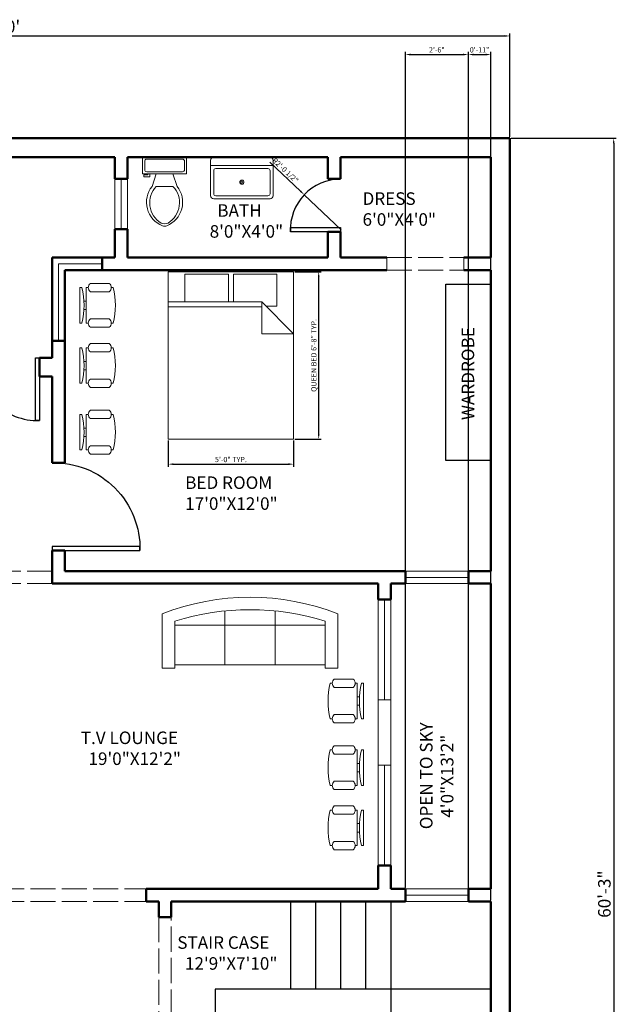
# Model space of a CAD drawing. Units: inches. Extents: x 2690 to 3266, y 1440 to 2261.
# Tile 4 of 4: x 2981 to 3266, y 1790 to 2261. Entities that reach past the tile are written whole.
import ezdxf

# ---------------------------------------------------------------- set-up
doc = ezdxf.new("R2010")
doc.units = ezdxf.units.IN
doc.linetypes.add('ACAD_ISO02W100', pattern=[15, 12, -3])
for name, color, linetype, lineweight in [('A-ANNO-DIMS', 2, 'Continuous', 18), ('A-ANNO-TEXT', 7, 'Continuous', 18), ('A-AREA-IDEN', 7, 'Continuous', 25), ('A-DOOR', 4, 'Continuous', 25), ('A-FLOR-CASE', 9, 'Continuous', 25), ('A-FLOR-FIXT', 9, 'Continuous', 18), ('A-FLOR-STRS', 7, 'Continuous', 25), ('A-FURN', 8, 'Continuous', 18), ('A-GLAZ', 3, 'Continuous', 18), ('A-WALL', 7, 'Continuous', 50), ('A-WALL-OVHD', 8, 'ACAD_ISO02W100', 18)]:
    doc.layers.add(name, color=color, linetype=linetype, lineweight=lineweight)
doc.styles.get("Standard").update_dxf_attribs({"font": 'arial.ttf'})
doc.dimstyles.new('ISO-25', dxfattribs={"dimtxt": 2.5, "dimasz": 2.5, "dimexe": 1.25, "dimexo": 0.625, "dimtad": 1, "dimlunit": 3, "dimtxsty": 'Standard', "dimcen": 2.5, "dimadec": 0, "dimazin": 0, "dimtfac": 1, "dimtmove": 0, "dimatfit": 3, "dimfxl": 1, "dimarcsym": 0})

# ---------------------------------------------------------------- blocks, each defined once
blk = doc.blocks.new('Toilet - top')
for p, q in [((9.5, -6), (9.5, -2)), ((-10, -8.5), (-8, -8.5)), ((-10, -9.5), (-10, -8.5)), ((-8, -8.5), (-8, -8)), ((-7, -8), (-7, -9.5)), ((-4, -8), (-6, -14)), ((4, -8), (6, -14)), ((-7, -9.5), (-10, -9.5)), ((4, -14), (-4, -14))]:
    blk.add_line(p, q)
blk.add_lwpolyline([(10.5, -8), (10.5, 0), (-10.5, 0), (-10.5, -8)], close=True)
for points in [[(-9.5, -2), (-9.5, -6)], [(8.5, -1), (-8.5, -1)], [(-8.5, -7), (8.5, -7)]]:
    blk.add_lwpolyline(points)
for centre, radius, start, end in [((-8.62, -1.88), 0.884, 81.8699, 188.1301), ((8.62, -1.88), 0.884, 351.8699, 98.1301), ((-8.62, -6.12), 0.884, 171.8699, 278.1301), ((8.62, -6.12), 0.884, 261.8699, 8.1301), ((3.52, -21.58), 12.17, 141.4691, 247.9714), ((4.2, -21.82), 11.33, 136.3677, 238.9468), ((-3.52, -21.58), 12.17, 292.0284, 38.5307), ((-4.2, -21.82), 11.33, 301.053, 43.6321), ((0, -27.88), 4, 245.7318, 294.2682), ((0, -29), 4, 254.8605, 285.1395)]:
    blk.add_arc(centre, radius, start, end)
blk = doc.blocks.new('Sink-single - 30 in top')
blk.add_line((-15, -3.999996), (15, -3.999996))
for points in [[(-13.5, 0), (13.5, 0)], [(-15, -18.499996), (-15, -1.5)], [(15, -1.5), (15, -18.499996)], [(-13.5, -17.499996), (-13.5, -6.499996)], [(-12.5, -5.499996), (12.5, -5.499996)], [(13.5, -6.499996), (13.5, -17.499996)], [(12.5, -18.499996), (-12.5, -18.499996)], [(13.5, -19.999996), (-13.5, -19.999996)]]:
    blk.add_lwpolyline(points)
for radius in [1, 0.5]:
    blk.add_circle((0, -11.999996), radius)
for centre, radius, start, end in [((-13.5, -1.5), 1.5, 90, 180), ((13.5, -1.5), 1.5, 0, 90), ((-12.5, -6.499996), 1, 90, 180), ((12.5, -6.499996), 1, 0, 90), ((-13.5, -18.499996), 1.5, 180, 270), ((-12.5, -17.499996), 1, 180, 270), ((12.5, -17.499996), 1, 270, 0), ((13.5, -18.499996), 1.5, 270, 0)]:
    blk.add_arc(centre, radius, start, end)
blk = doc.blocks.new('Sofa - Roundback 7 ft.')
for p, q in [((-12.00002, -32.4421), (-12.00003, -6.5971)), ((11.99997, -32.4421), (11.99998, -6.5971)), ((-36.000027, -34), (-36.000027, -11.4696)), ((-35.999844, -13.3819), (35.9998, -13.3819)), ((35.99998, -34), (35.99998, -11.4696)), ((-36.000027, -32.4421), (35.99998, -32.4421))]:
    blk.add_line(p, q)
for points in [[(-36.000027, -34), (-42.000027, -34), (-42.000027, -8)], [(41.99998, -8), (41.99998, -34), (35.99998, -34)]]:
    blk.add_lwpolyline(points)
for centre, radius, start, end in [((0, -114.25), 114.25, 68.43141, 111.5686), ((-0.00001, -127.1968), 121.1968, 72.72033, 107.2797)]:
    blk.add_arc(centre, radius, start, end)
blk = doc.blocks.new('Chair - Desk')
for p, q in [((-8.5, 0), (-8.5, -1)), ((-8.5, 0), (8.5, 0)), ((8.5, 0), (8.5, -1)), ((-8.5, -3), (-8.5, -4)), ((-8.5, -3), (8.5, -3)), ((-2, -3), (-2, -1.9355)), ((2, -1.9576), (2, -3)), ((8.5, -3), (8.5, -4)), ((-10.5, -5), (-10.5, -14)), ((-6.5, -14), (-6.5, -5)), ((6.5, -5), (6.5, -14)), ((10.5, -14), (10.5, -5)), ((-8.5, -15), (-8.5, -16)), ((8.5, -15), (8.5, -16))]:
    blk.add_line(p, q)
for centre, radius, start, end in [((-8.5, -6.5), 2.5, 36.8699, 143.1301), ((0, 34.625), 36.625, 256.5803, 283.4197), ((8.5, -6.5), 2.5, 36.8699, 143.1301), ((-8.5, -12.5), 2.5, 216.8699, 323.1301), ((8.5, -12.5), 2.5, 216.8699, 323.1301), ((0, 19.625), 36.625, 256.5803, 283.4197)]:
    blk.add_arc(centre, radius, start, end)
blk = doc.blocks.new('Bed - Queen')
for p, q in [((0, -80.00003), (0, 0)), ((0, 0), (59.99999, 0)), ((59.99999, 0), (59.99999, -80.00003)), ((7.99999, -1.2), (28.79998, -1.2)), ((7.99999, -14.4), (7.99999, -1.2)), ((28.79998, -1.2), (28.79998, -14.4)), ((31.19999, -1.2), (51.99999, -1.2)), ((31.19999, -14.4), (31.19999, -1.2)), ((51.99999, -1.2), (51.99999, -16.4)), ((0, -14.4), (44.8, -14.4)), ((44.8, -16.8), (0, -16.8)), ((59.99999, -29.6), (44.8, -14.4)), ((44.8, -14.4), (44.8, -29.6)), ((51.99999, -16.4), (46.79936, -16.4)), ((44.8, -29.6), (59.99999, -29.6)), ((59.99999, -80.00003), (0, -80.00003))]:
    blk.add_line(p, q)
blk = doc.blocks.new('*D12')
at = {"layer": 'A-ANNO-DIMS', "color": 0, "lineweight": -2, "transparency": 16777216}
for p, q in [((2735.48, 2205.11), (2735.48, 2254.67)), ((2737.98, 2253.42), (3212.98, 2253.42)), ((3215.48, 2205.11), (3215.48, 2254.67))]:
    blk.add_line(p, q, dxfattribs=at)
at = {"layer": 'A-ANNO-DIMS', "color": 0, "transparency": 16777216}
for points in [[(2737.98, 2253.84), (2737.98, 2253.01), (2735.48, 2253.42)], [(3212.98, 2253.84), (3212.98, 2253.01), (3215.48, 2253.42)]]:
    blk.add_solid(points, dxfattribs=at)
at = {"layer": 'Defpoints', "color": 0, "transparency": 16777216}
for p in [(3215.48, 2253.42), (2735.48, 2204.49), (3215.48, 2204.49)]:
    blk.add_point(p, dxfattribs=at)
at = {"layer": 'A-ANNO-DIMS', "color": 0, "transparency": 16777216, "insert": (2975.48, 2257.11), "char_height": 6, "attachment_point": 5}
blk.add_mtext("40'", dxfattribs=at)
blk = doc.blocks.new('*D15')
at = {"layer": 'A-ANNO-DIMS', "color": 0, "lineweight": -2, "transparency": 16777216}
for p, q in [((3216.1, 2204.49), (3266.46, 2204.49)), ((3265.21, 2201.99), (3265.21, 1483.99)), ((3216.1, 1481.49), (3266.46, 1481.49))]:
    blk.add_line(p, q, dxfattribs=at)
at = {"layer": 'A-ANNO-DIMS', "color": 0, "transparency": 16777216}
for points in [[(3264.79, 2201.99), (3265.63, 2201.99), (3265.21, 2204.49)], [(3264.79, 1483.99), (3265.63, 1483.99), (3265.21, 1481.49)]]:
    blk.add_solid(points, dxfattribs=at)
at = {"layer": 'Defpoints', "color": 0, "transparency": 16777216}
for p in [(3215.48, 2204.49), (3215.48, 1481.49), (3265.21, 1481.49)]:
    blk.add_point(p, dxfattribs=at)
at = {"layer": 'A-ANNO-DIMS', "color": 0, "transparency": 16777216, "insert": (3261.52, 1842.99), "char_height": 6, "attachment_point": 5, "rotation": 90}
blk.add_mtext('60\'-3"', dxfattribs=at)
blk = doc.blocks.new('DOOR-SWING-30IN')
for p, q in [((-2, -30), (-2, 0)), ((-2, 0), (0, 0)), ((0, 0), (0, -30)), ((0, -30), (-2, -30))]:
    blk.add_line(p, q)
blk.add_arc((-1, -1), 29.02, 178.0251, 271.9749)
blk = doc.blocks.new('DOOR-SWING-42IN')
for p, q in [((-42, 0), (-42, 2)), ((-42, 2), (0, 2)), ((0, 0), (-42, 0)), ((0, 2), (0, 0))]:
    blk.add_line(p, q)
blk.add_arc((-1, 1), 41.01, 88.6028, 181.3972)
blk = doc.blocks.new('WIN-24IN')
for p, q in [((0, 24), (0, 0)), ((3, 0), (3, 24)), ((3, 24), (6, 24)), ((6, 24), (6, 0)), ((0, 0), (3, 0))]:
    blk.add_line(p, q)
blk = doc.blocks.new('WARDROBE-PLAN')
blk.add_lwpolyline([(0, 0), (21.23, 0), (21.23, -84.36), (0, -84.36)], close=True)
blk = doc.blocks.new('*D29')
at = {"layer": 'A-ANNO-DIMS', "color": 0, "lineweight": -2, "transparency": 16777216}
for p, q in [((3112.66, 2140.62), (3125.28, 2140.62)), ((3124.03, 2063.12), (3124.03, 2138.12)), ((3112.66, 2060.62), (3125.28, 2060.62))]:
    blk.add_line(p, q, dxfattribs=at)
at = {"layer": 'A-ANNO-DIMS', "color": 0, "transparency": 16777216}
for points in [[(3123.61, 2138.12), (3124.45, 2138.12), (3124.03, 2140.62)], [(3123.61, 2063.12), (3124.45, 2063.12), (3124.03, 2060.62)]]:
    blk.add_solid(points, dxfattribs=at)
at = {"layer": 'Defpoints', "color": 0, "transparency": 16777216}
for p in [(3112.03, 2140.62), (3124.03, 2140.62), (3112.03, 2060.62)]:
    blk.add_point(p, dxfattribs=at)
at = {"layer": 'A-ANNO-DIMS', "color": 0, "transparency": 16777216, "insert": (3122.04, 2100.62), "char_height": 2.5, "attachment_point": 5, "rotation": 90}
blk.add_mtext('QUEEN BED 6\'-8" TYP.', dxfattribs=at)
blk = doc.blocks.new('*D30')
at = {"layer": 'A-ANNO-DIMS', "color": 0, "lineweight": -2, "transparency": 16777216}
for p, q in [((3052.03, 2059.99), (3052.03, 2047.37)), ((3112.03, 2059.99), (3112.03, 2047.37)), ((3054.53, 2048.62), (3109.53, 2048.62))]:
    blk.add_line(p, q, dxfattribs=at)
at = {"layer": 'A-ANNO-DIMS', "color": 0, "transparency": 16777216}
for points in [[(3054.53, 2049.03), (3054.53, 2048.2), (3052.03, 2048.62)], [(3109.53, 2049.03), (3109.53, 2048.2), (3112.03, 2048.62)]]:
    blk.add_solid(points, dxfattribs=at)
at = {"layer": 'Defpoints', "color": 0, "transparency": 16777216}
for p in [(3052.03, 2060.62), (3112.03, 2060.62), (3112.03, 2048.62)]:
    blk.add_point(p, dxfattribs=at)
at = {"layer": 'A-ANNO-DIMS', "color": 0, "transparency": 16777216, "insert": (3082.03, 2050.52), "char_height": 2.5, "attachment_point": 5}
blk.add_mtext('5\'-0" TYP.', dxfattribs=at)
blk = doc.blocks.new('*D58')
at = {"layer": 'A-ANNO-DIMS', "color": 0, "lineweight": -2, "transparency": 16777216}
for p, q in [((3165.5, 1846.11), (3165.5, 2245.79)), ((3168, 2244.54), (3193.15, 2244.54)), ((3195.65, 1846.11), (3195.65, 2245.79))]:
    blk.add_line(p, q, dxfattribs=at)
at = {"layer": 'A-ANNO-DIMS', "color": 0, "transparency": 16777216}
for points in [[(3168, 2244.95), (3168, 2244.12), (3165.5, 2244.54)], [(3193.15, 2244.95), (3193.15, 2244.12), (3195.65, 2244.54)]]:
    blk.add_solid(points, dxfattribs=at)
at = {"layer": 'Defpoints', "color": 0, "transparency": 16777216}
for p in [(3195.65, 2244.54), (3165.5, 1845.49), (3195.65, 1845.49)]:
    blk.add_point(p, dxfattribs=at)
at = {"layer": 'A-ANNO-DIMS', "color": 0, "transparency": 16777216, "insert": (3180.57, 2246.44), "char_height": 2.5, "attachment_point": 5}
blk.add_mtext('2\'-6"', dxfattribs=at)
blk = doc.blocks.new('*D59')
at = {"layer": 'A-ANNO-DIMS', "color": 0, "lineweight": -2, "transparency": 16777216}
for p, q in [((3195.65, 1840.11), (3195.65, 2245.79)), ((3198.15, 2244.54), (3203.98, 2244.54)), ((3206.48, 1840.11), (3206.48, 2245.79))]:
    blk.add_line(p, q, dxfattribs=at)
at = {"layer": 'A-ANNO-DIMS', "color": 0, "transparency": 16777216}
for points in [[(3198.15, 2244.95), (3198.15, 2244.12), (3195.65, 2244.54)], [(3203.98, 2244.95), (3203.98, 2244.12), (3206.48, 2244.54)]]:
    blk.add_solid(points, dxfattribs=at)
at = {"layer": 'Defpoints', "color": 0, "transparency": 16777216}
for p in [(3206.48, 2244.54), (3195.65, 1839.49), (3206.48, 1839.49)]:
    blk.add_point(p, dxfattribs=at)
at = {"layer": 'A-ANNO-DIMS', "color": 0, "transparency": 16777216, "insert": (3201.06, 2246.44), "char_height": 2.5, "attachment_point": 5}
blk.add_mtext('0\'-11"', dxfattribs=at)
blk = doc.blocks.new('*D62')
at = {"layer": 'A-ANNO-DIMS', "color": 0, "lineweight": -2, "transparency": 16777216}
for p, q in [((3100.7, 2193.04), (3115.31, 2179.18)), ((3134.76, 2160.74), (3117.13, 2177.46))]:
    blk.add_line(p, q, dxfattribs=at)
at = {"layer": 'A-ANNO-DIMS', "color": 0, "transparency": 16777216}
blk.add_solid([(3115.6, 2179.49), (3115.03, 2178.88), (3117.13, 2177.46)], dxfattribs=at)
at = {"layer": 'Defpoints', "color": 0, "transparency": 16777216}
for p in [(3117.13, 2177.46), (3134.76, 2160.74)]:
    blk.add_point(p, dxfattribs=at)
at = {"layer": 'A-ANNO-DIMS', "color": 0, "transparency": 16777216, "insert": (3107.87, 2188.89), "char_height": 2.5, "attachment_point": 5, "rotation": 316.5144}
blk.add_mtext('R2\'-0 1/2"', dxfattribs=at)

msp = doc.modelspace()

# ---------------------------------------------------------------- linework, layer by layer
at = {"layer": 'A-DOOR'}
for p, q in [((3110.476, 2159.738), (3110.476, 2161.738)), ((3110.476, 2161.738), (3134.476, 2161.738)), ((3134.476, 2161.738), (3134.476, 2159.738)), ((3134.476, 2159.738), (3110.476, 2159.738))]:
    msp.add_line(p, q, dxfattribs=at)
msp.add_arc((3134.76, 2160.738), 24.304, 90.66918, 182.35809, dxfattribs=at)
at = {"layer": 'A-FLOR-STRS'}
for p, q in [((3110.476, 1839.486), (3110.476, 1797.486)), ((3122.476, 1839.486), (3122.476, 1797.486)), ((3134.476, 1839.486), (3134.476, 1797.486)), ((3146.476, 1839.486), (3146.476, 1797.486)), ((3158.476, 1839.486), (3158.476, 1745.486)), ((3206.476, 1797.486), (3074.476, 1797.486)), ((3074.476, 1797.486), (3074.476, 1745.486))]:
    msp.add_line(p, q, dxfattribs=at)
at = {"layer": 'A-GLAZ'}
for p, q in [((2999.476, 2107.646), (2999.476, 2144.486)), ((2999.476, 2144.486), (3020.476, 2144.486)), ((3165.496, 1994.486), (3165.496, 1997.486)), ((3165.496, 1997.486), (3195.653, 1997.486)), ((3165.496, 1991.486), (3165.496, 1997.486)), ((3195.653, 1997.486), (3195.653, 1991.486)), ((3195.653, 1994.486), (3165.496, 1994.486)), ((3195.653, 1991.486), (3195.653, 1994.486)), ((3165.496, 1991.486), (3195.653, 1991.486)), ((3195.653, 1991.486), (3165.496, 1991.486)), ((3152.476, 1983.961), (3152.476, 1856.641)), ((3158.476, 1983.961), (3152.476, 1983.961)), ((3155.476, 1935.961), (3155.476, 1983.961)), ((3158.476, 1856.641), (3158.476, 1983.961)), ((3158.476, 1935.961), (3152.476, 1935.961)), ((3152.476, 1904.641), (3158.476, 1904.641)), ((3155.476, 1904.641), (3155.476, 1856.641)), ((3152.476, 1856.641), (3158.476, 1856.641)), ((3165.496, 1842.486), (3165.496, 1845.486)), ((3165.496, 1845.486), (3195.653, 1845.486)), ((3195.137, 1842.486), (3165.496, 1842.486)), ((3195.653, 1842.486), (3195.137, 1842.486)), ((3195.653, 1839.486), (3195.653, 1842.486)), ((3165.496, 1839.486), (3195.653, 1839.486))]:
    msp.add_line(p, q, dxfattribs=at)
at = {"layer": 'A-WALL'}
for p, q in [((2735.476, 2204.486), (3215.476, 2204.486)), ((3215.476, 2204.486), (3215.476, 1538.486)), ((2870.476, 2195.486), (3026.476, 2195.486)), ((3026.476, 2195.486), (3026.476, 2185.041)), ((3032.476, 2195.486), (3032.476, 2185.041)), ((3032.476, 2195.486), (3128.476, 2195.486)), ((3128.476, 2195.486), (3128.476, 2185.041)), ((3134.476, 2195.486), (3134.476, 2185.041)), ((3134.476, 2195.486), (3206.476, 2195.486)), ((3206.476, 2195.486), (3206.476, 2147.486)), ((3026.476, 2185.041), (3032.476, 2185.041)), ((3128.476, 2185.041), (3134.476, 2185.041)), ((3026.476, 2161.041), (3032.476, 2161.041)), ((3026.476, 2161.041), (3026.476, 2147.486)), ((3032.476, 2161.041), (3032.476, 2147.486)), ((3128.476, 2159.738), (3128.476, 2147.486)), ((3128.476, 2159.738), (3134.476, 2159.738)), ((3134.476, 2159.738), (3134.476, 2147.486)), ((3020.476, 2147.486), (2996.476, 2147.486)), ((2996.476, 2147.486), (2996.476, 2141.486)), ((3020.476, 2141.486), (3020.476, 2147.486)), ((3020.476, 2147.486), (3026.476, 2147.486)), ((3020.476, 2141.486), (3020.476, 2147.486)), ((3032.476, 2147.486), (3128.476, 2147.486)), ((3134.476, 2147.486), (3156.656, 2147.486)), ((3193.502, 2147.486), (3206.476, 2147.486)), ((2996.476, 2141.486), (2996.476, 2099.486)), ((3002.476, 2141.486), (3002.476, 2049.268)), ((3002.476, 2141.486), (3020.476, 2141.486)), ((3026.476, 2141.486), (3020.476, 2141.486)), ((3026.476, 2141.486), (3156.656, 2141.486)), ((3193.502, 2141.486), (3206.476, 2141.486)), ((3206.476, 2141.486), (3206.476, 1997.486)), ((2996.476, 2107.646), (3002.476, 2107.646)), ((2990.461, 2099.486), (2990.461, 2090.486)), ((2990.461, 2099.486), (2996.476, 2099.486)), ((2990.461, 2090.486), (2996.476, 2090.486)), ((2996.476, 2090.486), (2996.476, 2049.268)), ((2996.476, 2049.268), (3002.476, 2049.268)), ((2996.476, 2007.268), (3002.476, 2007.268)), ((2996.476, 2007.268), (2996.476, 1991.486)), ((3002.476, 2007.268), (3002.476, 1997.486)), ((3002.476, 1997.486), (3165.496, 1997.486)), ((3165.496, 1997.486), (3165.496, 1991.486)), ((3195.653, 1997.486), (3195.653, 1991.486)), ((3195.653, 1997.486), (3206.476, 1997.486)), ((2996.476, 1991.486), (3152.476, 1991.486)), ((3152.476, 1991.486), (3152.476, 1983.961)), ((3158.476, 1991.486), (3158.476, 1983.961)), ((3158.476, 1991.486), (3165.496, 1991.486)), ((3195.653, 1991.486), (3206.476, 1991.486)), ((3206.476, 1991.486), (3206.476, 1845.486)), ((3152.476, 1983.961), (3158.476, 1983.961)), ((3152.476, 1856.641), (3158.476, 1856.641)), ((3152.476, 1856.641), (3152.476, 1845.486)), ((3158.476, 1856.641), (3158.476, 1845.486)), ((3041.476, 1839.486), (3041.476, 1845.486)), ((3041.476, 1845.486), (3047.476, 1845.486)), ((3152.476, 1845.486), (3041.476, 1845.486)), ((3165.496, 1845.486), (3158.476, 1845.486)), ((3165.496, 1845.486), (3165.496, 1839.486)), ((3206.476, 1845.486), (3195.653, 1845.486)), ((3195.653, 1845.486), (3195.653, 1839.486)), ((3047.476, 1839.486), (3041.476, 1839.486)), ((3047.476, 1839.486), (3041.476, 1839.486)), ((3047.476, 1839.486), (3047.476, 1831.977)), ((3053.476, 1839.486), (3053.476, 1831.977)), ((3165.496, 1839.486), (3053.476, 1839.486)), ((3206.476, 1839.486), (3195.653, 1839.486)), ((3206.476, 1839.486), (3206.476, 1745.486)), ((3047.476, 1831.977), (3053.476, 1831.977))]:
    msp.add_line(p, q, dxfattribs=at)
at = {"layer": 'A-WALL-OVHD'}
for p, q in [((3156.656, 2147.486), (3156.656, 2141.486)), ((3156.656, 2147.486), (3193.502, 2147.486)), ((3193.502, 2147.486), (3193.502, 2141.486)), ((3156.656, 2141.486), (3193.502, 2141.486)), ((2996.476, 1997.486), (2924.476, 1997.486)), ((2924.476, 1991.486), (2996.476, 1991.486)), ((2926.112, 1845.486), (3041.476, 1845.486)), ((2926.112, 1839.486), (3041.476, 1839.486)), ((3047.476, 1831.977), (3047.476, 1755.439)), ((3053.476, 1755.439), (3053.476, 1831.977))]:
    msp.add_line(p, q, dxfattribs=at)

# ---------------------------------------------------------------- block references
at = {"layer": 'A-DOOR'}
msp.add_blockref('DOOR-SWING-30IN', (2990.461, 2099.486), dxfattribs=at)
at = {"layer": 'A-DOOR', "extrusion": (0, 0, -1), "zscale": -1}
msp.add_blockref('DOOR-SWING-42IN', (-2996.476, 2007.268), dxfattribs=at)
at = {"layer": 'A-FLOR-CASE'}
msp.add_blockref('WARDROBE-PLAN', (3184.869, 2134.74), dxfattribs=at)
at = {"layer": 'A-FLOR-FIXT'}
for name, p in [('Toilet - top', (3050.281, 2195.486)), ('Sink-single - 30 in top', (3087.267, 2195.486))]:
    msp.add_blockref(name, p, dxfattribs=at)
at = {"layer": 'A-FURN'}
for name, p in [('Bed - Queen', (3052.031, 2140.618)), ('Sofa - Roundback 7 ft.', (3091.171, 1985.016))]:
    msp.add_blockref(name, p, dxfattribs=at)
for p, rotation in [((3009.75, 2124.592), 89.99999999999999), ((3009.75, 2095.798), 89.99999999999999), ((3009.75, 2063.92), 89.99999999999999), ((3145.503, 1935.361), 270), ((3145.503, 1903.482), 270), ((3145.503, 1874.689), 270)]:
    msp.add_blockref('Chair - Desk', p, dxfattribs=dict(at, rotation=rotation))
at = {"layer": 'A-GLAZ', "rotation": 180}
msp.add_blockref('WIN-24IN', (3032.476, 2185.041), dxfattribs=at)

# ---------------------------------------------------------------- texts
at = {"layer": 'A-ANNO-TEXT', "insert": (3192.448, 2064.22), "char_height": 6, "attachment_point": 1, "rotation": 90}
msp.add_mtext_dynamic_manual_height_columns('   WARDROBE', width=77.52183, gutter_width=12.5, heights=[0], dxfattribs=at)
at = {"layer": 'A-AREA-IDEN', "char_height": 6, "attachment_point": 1}
for s, insert in [('      DRESS\\P      6\'0"X4\'0"', (3134.018, 2178.64)), ('      BATH\\P    8\'0"X4\'0"', (3064.515, 2172.943)), ('      BED ROOM\\P      17\'0"X12\'0"', (3049.135, 2042.772)), (' T.V LOUNGE\\P   19\'0"X12\'2"', (3008.354, 1920.754)), (' STAIR CASE\\P   12\'9"X7\'10"', (3054.532, 1822.837))]:
    msp.add_mtext_dynamic_manual_height_columns(s, width=77.52183, gutter_width=12.5, heights=[0], dxfattribs=dict(at, insert=insert))
at = {"layer": 'A-AREA-IDEN', "insert": (3172.493, 1870.352), "char_height": 6, "attachment_point": 1, "rotation": 90}
msp.add_mtext_dynamic_manual_height_columns('  OPEN TO SKY\\P     4\'0"X13\'2"', width=77.52183, gutter_width=12.5, heights=[0], dxfattribs=at)

# ---------------------------------------------------------------- dimensions: what is measured, and where the dimension line sits
at = {"layer": 'A-ANNO-DIMS'}
for base, p1, p2, override, picture, middle in [((3215.476, 2253.424), (2735.476, 2204.486), (3215.476, 2204.486), {"dimtxt": 6, "dimclrd": 0, "dimclre": 0, "dimclrt": 0}, '*D12', (2975.476, 2257.113)), ((3195.653, 2244.536), (3165.496, 1845.486), (3195.653, 1845.486), {"dimdec": 1, "dimlfac": 1, "dimrnd": 0, "dimzin": 1, "dimdsep": 46, "dimlunit": 4, "dimfrac": 2}, '*D58', (3180.575, 2246.437)), ((3206.476, 2244.536), (3195.653, 1839.486), (3206.476, 1839.486), {"dimdec": 1, "dimlfac": 1, "dimrnd": 0, "dimzin": 1, "dimdsep": 46, "dimlunit": 4, "dimfrac": 2}, '*D59', (3201.065, 2246.437))]:
    dim = msp.add_linear_dim(base=base, p1=p1, p2=p2, dimstyle='ISO-25', override=override, dxfattribs=at)
    dim.commit()
    dim.dimension.update_dxf_attribs({"geometry": picture, "text_midpoint": middle})
dim = msp.add_linear_dim(base=(3265.21, 1481.486), p1=(3215.476, 2204.486), p2=(3215.476, 1481.486), angle=90, dimstyle='ISO-25', override={"dimtxt": 6, "dimclrd": 0, "dimclre": 0, "dimclrt": 0}, dxfattribs=at)
dim.commit()
dim.dimension.update_dxf_attribs({"geometry": '*D15', "text_midpoint": (3261.519, 1842.986)})
dim = msp.add_radius_dim(center=(3134.76, 2160.738), mpoint=(3117.126, 2177.464), dimstyle='ISO-25', override={"dimdec": 1, "dimlfac": 1, "dimrnd": 0, "dimzin": 1, "dimdsep": 46, "dimlunit": 4, "dimfrac": 2}, dxfattribs=at)
dim.commit()
dim.dimension.update_dxf_attribs({"geometry": '*D62', "text_midpoint": (3106.546, 2187.499), "dimtype": 164})
dim = msp.add_linear_dim(base=(3124.031, 2140.618), p1=(3112.031, 2060.618), p2=(3112.031, 2140.618), angle=90, text='QUEEN BED <> TYP.', dimstyle='ISO-25', override={"dimdec": 1, "dimlfac": 1, "dimrnd": 0, "dimzin": 1, "dimdsep": 46, "dimlunit": 4, "dimfrac": 2}, dxfattribs=at)
dim.commit()
dim.dimension.update_dxf_attribs({"geometry": '*D29', "text_midpoint": (3122.037, 2100.618)})
dim = msp.add_linear_dim(base=(3112.031, 2048.618), p1=(3052.031, 2060.618), p2=(3112.031, 2060.618), text='<> TYP.', dimstyle='ISO-25', override={"dimdec": 1, "dimlfac": 1, "dimrnd": 0, "dimzin": 1, "dimdsep": 46, "dimlunit": 4, "dimfrac": 2}, dxfattribs=at)
dim.commit()
dim.dimension.update_dxf_attribs({"geometry": '*D30', "text_midpoint": (3082.031, 2050.52)})

doc.saveas('drawing.dxf')
